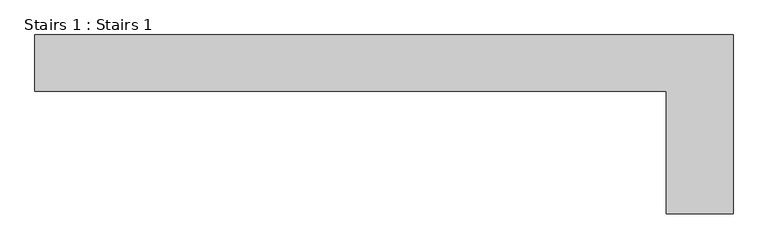
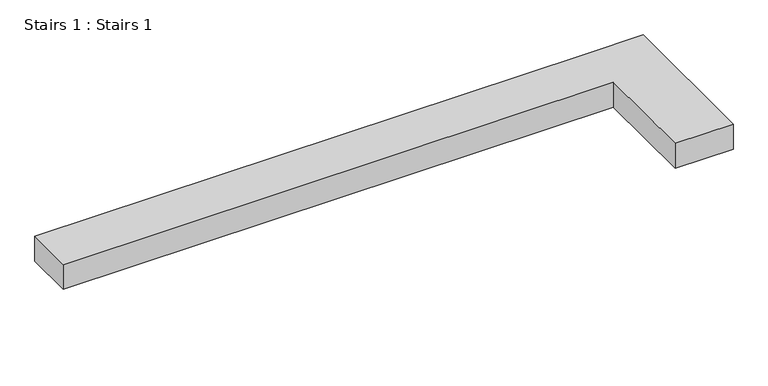
"""IFC4 building model written with IfcOpenShell, lengths in millimetres: stair geometry, Stairs 1 : Stairs 1."""

from ifc_helpers import new_model, si_unit, origin, origin_with_axes, place, context, project, spatial, polyline, outline, extrude, source, transform, mapped, element, save


def stairs_1_stairs_1_bf5218fc(model_context):
    return source(origin(), model_context, "Body", "SweptSolid", [
        extrude(outline(polyline([(-48002.6209459, 28071.8116741), (-47672.4209459, 28071.8116741), (-47672.4209459, 27185.8922457), (-48002.6209459, 27185.8922457), (-48002.6209459, 27792.4116741), (-51132.7755215, 27792.4116741), (-51132.7755215, 28071.8116741), (-48002.6209459, 28071.8116741)])), origin_with_axes(), (0.0, 0.0, 1.0), 150.01875),
    ])


if __name__ == "__main__":
    model = new_model("IFC4")
    model_context = context("Model", 3, world=origin())
    ifc_project = project(units=[si_unit("LENGTHUNIT", "METRE", prefix="MILLI")], contexts=[model_context])
    site = spatial("IfcSite", under=ifc_project)
    building = spatial("IfcBuilding", under=site)
    placement = place(None, origin())
    stairs_1_stairs_1_shape = stairs_1_stairs_1_bf5218fc(model_context)
    element("IfcStair", 1, ObjectType="Stairs 1 : Stairs 1", at=placement, inside=building, context=model_context, shape_type="MappedRepresentation", body=[
        mapped(stairs_1_stairs_1_shape, transform((0.0, 0.0, 0.0), x_axis=(1.0, 0.0, 0.0), y_axis=(0.0, 1.0, 0.0), z_axis=(0.0, 0.0, 1.0))),
    ])
    save(model, "model.ifc")
